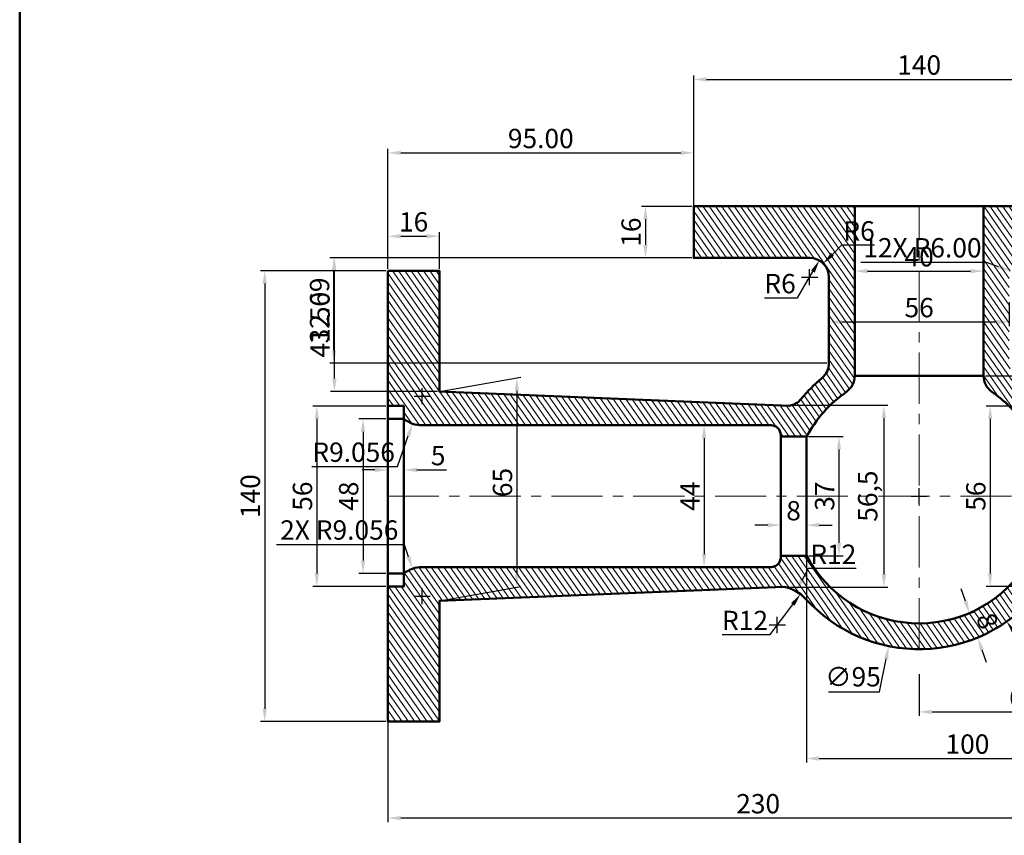
# Model space of a CAD drawing. Units: millimetres. Extents: x 39 to 520, y -165 to 464.
# Tile 2 of 4: x 39 to 345, y -9 to 244. Entities that reach past the tile are written whole.
import ezdxf

# ---------------------------------------------------------------- set-up
doc = ezdxf.new("R2010")
doc.units = ezdxf.units.MM
doc.header["$LTSCALE"] = 0.5
doc.linetypes.add('CENTER', pattern=[50.8, 31.75, -6.35, 6.35, -6.35])
for name, color, linetype, lineweight in [('M-CNTR', 1, 'CENTER', 18), ('M-DIMS', 2, 'Continuous', 25), ('M-HATC', 8, 'Continuous', 18), ('M-OUTL', 7, 'Continuous', 50), ('M-TTLB', 7, 'Continuous', 50)]:
    doc.layers.add(name, color=color, linetype=linetype, lineweight=lineweight)
doc.styles.get("Standard").update_dxf_attribs({"font": 'arial.ttf'})
doc.dimstyles.new('ISO-25', dxfattribs={"dimtxt": 6, "dimasz": 4, "dimexe": 1.25, "dimexo": 0.625, "dimtad": 1, "dimtoh": 1, "dimdec": 1, "dimtxsty": 'Standard', "dimcen": 2.5, "dimadec": 0, "dimazin": 0, "dimtfac": 1, "dimtdec": 1, "dimtofl": 0, "dimtmove": 0, "dimatfit": 3, "dimfxl": 1, "dimarcsym": 0})

# ---------------------------------------------------------------- blocks, each defined once
blk = doc.blocks.new('*D1')
at = {"layer": 'Defpoints', "color": 0, "ltscale": 0.5, "transparency": 16777216}
for p in [(388.62, 225.52), (248.62, 186.1), (388.62, 186.1)]:
    blk.add_point(p, dxfattribs=at)
at = {"layer": 'M-DIMS', "color": 0, "lineweight": -2, "ltscale": 0.5, "transparency": 16777216}
for p, q in [((248.62, 186.73), (248.62, 226.77)), ((388.62, 186.73), (388.62, 226.77)), ((252.62, 225.52), (384.62, 225.52))]:
    blk.add_line(p, q, dxfattribs=at)
at = {"layer": 'M-DIMS', "color": 0, "ltscale": 0.5, "transparency": 16777216}
for points in [[(252.62, 226.18), (252.62, 224.85), (248.62, 225.52)], [(384.62, 226.18), (384.62, 224.85), (388.62, 225.52)]]:
    blk.add_solid(points, dxfattribs=at)
at = {"layer": 'M-DIMS', "color": 0, "ltscale": 0.5, "transparency": 16777216, "insert": (318.62, 229.21), "char_height": 6, "attachment_point": 5}
blk.add_mtext('140', dxfattribs=at)
blk = doc.blocks.new('*D2')
at = {"layer": 'Defpoints', "color": 0, "ltscale": 0.5, "transparency": 16777216}
for p in [(290.62, 156.95), (346.62, 156.95), (346.62, 150.19)]:
    blk.add_point(p, dxfattribs=at)
at = {"layer": 'M-DIMS', "color": 0, "lineweight": -2, "ltscale": 0.5, "transparency": 16777216}
for p, q in [((290.62, 156.32), (290.62, 148.94)), ((346.62, 156.32), (346.62, 148.94)), ((294.62, 150.19), (342.62, 150.19))]:
    blk.add_line(p, q, dxfattribs=at)
at = {"layer": 'M-DIMS', "color": 0, "ltscale": 0.5, "transparency": 16777216}
for points in [[(294.62, 150.85), (294.62, 149.52), (290.62, 150.19)], [(342.62, 150.85), (342.62, 149.52), (346.62, 150.19)]]:
    blk.add_solid(points, dxfattribs=at)
at = {"layer": 'M-DIMS', "color": 0, "ltscale": 0.5, "transparency": 16777216, "insert": (318.62, 153.88), "char_height": 6, "attachment_point": 5}
blk.add_mtext('56', dxfattribs=at)
blk = doc.blocks.new('*D3')
at = {"layer": 'Defpoints', "color": 0, "ltscale": 0.5, "transparency": 16777216}
for p in [(298.62, 172.66), (338.62, 172.66), (338.62, 165.99)]:
    blk.add_point(p, dxfattribs=at)
at = {"layer": 'M-DIMS', "color": 0, "lineweight": -2, "ltscale": 0.5, "transparency": 16777216}
for p, q in [((298.62, 172.04), (298.62, 164.74)), ((338.62, 172.04), (338.62, 164.74)), ((302.62, 165.99), (334.62, 165.99))]:
    blk.add_line(p, q, dxfattribs=at)
at = {"layer": 'M-DIMS', "color": 0, "ltscale": 0.5, "transparency": 16777216}
for points in [[(302.62, 166.65), (302.62, 165.32), (298.62, 165.99)], [(334.62, 166.65), (334.62, 165.32), (338.62, 165.99)]]:
    blk.add_solid(points, dxfattribs=at)
at = {"layer": 'M-DIMS', "color": 0, "ltscale": 0.5, "transparency": 16777216, "insert": (318.62, 169.67), "char_height": 6, "attachment_point": 5}
blk.add_mtext('40', dxfattribs=at)
blk = doc.blocks.new('*D5')
at = {"layer": 'Defpoints', "color": 0, "ltscale": 0.5, "transparency": 16777216}
for p in [(248.62, 186.1), (233.62, 170.1), (248.62, 170.1)]:
    blk.add_point(p, dxfattribs=at)
at = {"layer": 'M-DIMS', "color": 0, "lineweight": -2, "ltscale": 0.5, "transparency": 16777216}
for p, q in [((248, 186.1), (232.37, 186.1)), ((233.62, 182.1), (233.62, 174.1)), ((248, 170.1), (232.37, 170.1))]:
    blk.add_line(p, q, dxfattribs=at)
at = {"layer": 'M-DIMS', "color": 0, "ltscale": 0.5, "transparency": 16777216}
for points in [[(232.96, 182.1), (234.29, 182.1), (233.62, 186.1)], [(232.96, 174.1), (234.29, 174.1), (233.62, 170.1)]]:
    blk.add_solid(points, dxfattribs=at)
at = {"layer": 'M-DIMS', "color": 0, "ltscale": 0.5, "transparency": 16777216, "insert": (229.94, 178.1), "char_height": 6, "attachment_point": 5, "rotation": 90}
blk.add_mtext('16', dxfattribs=at)
blk = doc.blocks.new('*D11')
at = {"layer": 'Defpoints', "color": 0, "ltscale": 0.5, "transparency": 16777216}
for p in [(318.62, 41.45), (383.62, 36.1), (383.62, 29.1)]:
    blk.add_point(p, dxfattribs=at)
at = {"layer": 'M-DIMS', "color": 0, "lineweight": -2, "ltscale": 0.5, "transparency": 16777216}
for p, q in [((318.62, 40.83), (318.62, 27.85)), ((383.62, 35.48), (383.62, 27.85)), ((322.62, 29.1), (379.62, 29.1))]:
    blk.add_line(p, q, dxfattribs=at)
at = {"layer": 'M-DIMS', "color": 0, "ltscale": 0.5, "transparency": 16777216}
for points in [[(322.62, 29.77), (322.62, 28.44), (318.62, 29.1)], [(379.62, 29.77), (379.62, 28.44), (383.62, 29.1)]]:
    blk.add_solid(points, dxfattribs=at)
at = {"layer": 'M-DIMS', "color": 0, "ltscale": 0.5, "transparency": 16777216, "insert": (351.12, 32.79), "char_height": 6, "attachment_point": 5}
blk.add_mtext('65', dxfattribs=at)
blk = doc.blocks.new('*D12')
at = {"layer": 'Defpoints', "color": 0, "ltscale": 0.5, "transparency": 16777216}
for p in [(283.62, 96.1), (383.62, 48.96), (383.62, 14.65)]:
    blk.add_point(p, dxfattribs=at)
at = {"layer": 'M-DIMS', "color": 0, "lineweight": -2, "ltscale": 0.5, "transparency": 16777216}
for p, q in [((283.62, 95.48), (283.62, 13.4)), ((383.62, 48.34), (383.62, 13.4)), ((287.62, 14.65), (379.62, 14.65))]:
    blk.add_line(p, q, dxfattribs=at)
at = {"layer": 'M-DIMS', "color": 0, "ltscale": 0.5, "transparency": 16777216}
for points in [[(287.62, 15.32), (287.62, 13.98), (283.62, 14.65)], [(379.62, 15.32), (379.62, 13.98), (383.62, 14.65)]]:
    blk.add_solid(points, dxfattribs=at)
at = {"layer": 'M-DIMS', "color": 0, "ltscale": 0.5, "transparency": 16777216, "insert": (333.62, 18.34), "char_height": 6, "attachment_point": 5}
blk.add_mtext('100', dxfattribs=at)
blk = doc.blocks.new('*D13')
at = {"layer": 'Defpoints', "color": 0, "ltscale": 0.5, "transparency": 16777216}
for p in [(153.62, 36.1), (383.62, 36.1), (153.62, -3.86)]:
    blk.add_point(p, dxfattribs=at)
at = {"layer": 'M-DIMS', "color": 0, "lineweight": -2, "ltscale": 0.5, "transparency": 16777216}
for p, q in [((153.62, 35.48), (153.62, -5.11)), ((383.62, 35.48), (383.62, -5.11)), ((379.62, -3.86), (157.62, -3.86))]:
    blk.add_line(p, q, dxfattribs=at)
at = {"layer": 'M-DIMS', "color": 0, "ltscale": 0.5, "transparency": 16777216}
for points in [[(157.62, -3.19), (157.62, -4.53), (153.62, -3.86)], [(379.62, -3.19), (379.62, -4.53), (383.62, -3.86)]]:
    blk.add_solid(points, dxfattribs=at)
at = {"layer": 'M-DIMS', "color": 0, "ltscale": 0.5, "transparency": 16777216, "insert": (268.62, -0.17), "char_height": 6, "attachment_point": 5}
blk.add_mtext('230', dxfattribs=at)
blk = doc.blocks.new('*D14')
at = {"layer": 'Defpoints', "color": 0, "ltscale": 0.5, "transparency": 16777216}
for p in [(359.93, 124.1), (340.68, 68.1), (362.28, 68.1)]:
    blk.add_point(p, dxfattribs=at)
at = {"layer": 'M-DIMS', "color": 0, "lineweight": -2, "ltscale": 0.5, "transparency": 16777216}
for p, q in [((359.3, 124.1), (339.43, 124.1)), ((340.68, 120.1), (340.68, 72.1)), ((361.65, 68.1), (339.43, 68.1))]:
    blk.add_line(p, q, dxfattribs=at)
at = {"layer": 'M-DIMS', "color": 0, "ltscale": 0.5, "transparency": 16777216}
for points in [[(340.02, 120.1), (341.35, 120.1), (340.68, 124.1)], [(340.02, 72.1), (341.35, 72.1), (340.68, 68.1)]]:
    blk.add_solid(points, dxfattribs=at)
at = {"layer": 'M-DIMS', "color": 0, "ltscale": 0.5, "transparency": 16777216, "insert": (337, 96.1), "char_height": 6, "attachment_point": 5, "rotation": 90}
blk.add_mtext('56', dxfattribs=at)
blk = doc.blocks.new('*D16')
at = {"layer": 'Defpoints', "color": 0, "ltscale": 0.5, "transparency": 16777216}
for p in [(283.62, 114.6), (283.72, 77.6), (293.73, 77.6)]:
    blk.add_point(p, dxfattribs=at)
at = {"layer": 'M-DIMS', "color": 0, "lineweight": -2, "ltscale": 0.5, "transparency": 16777216}
for p, q in [((284.25, 114.6), (294.98, 114.6)), ((293.73, 110.6), (293.73, 81.6)), ((284.35, 77.6), (294.98, 77.6))]:
    blk.add_line(p, q, dxfattribs=at)
at = {"layer": 'M-DIMS', "color": 0, "ltscale": 0.5, "transparency": 16777216}
for points in [[(293.07, 110.6), (294.4, 110.6), (293.73, 114.6)], [(293.07, 81.6), (294.4, 81.6), (293.73, 77.6)]]:
    blk.add_solid(points, dxfattribs=at)
at = {"layer": 'M-DIMS', "color": 0, "ltscale": 0.5, "transparency": 16777216, "insert": (290.04, 96.1), "char_height": 6, "attachment_point": 5, "rotation": 90}
blk.add_mtext('37', dxfattribs=at)
blk = doc.blocks.new('*D17')
at = {"layer": 'Defpoints', "color": 0, "ltscale": 0.5, "transparency": 16777216}
for p in [(275.62, 88.27), (275.62, 87.12), (283.62, 88.27)]:
    blk.add_point(p, dxfattribs=at)
at = {"layer": 'M-DIMS', "color": 0, "lineweight": -2, "ltscale": 0.5, "transparency": 16777216}
for p, q in [((271.62, 87.12), (267.62, 87.12)), ((275.62, 87.64), (275.62, 85.87)), ((283.62, 87.64), (283.62, 85.87)), ((287.62, 87.12), (291.62, 87.12))]:
    blk.add_line(p, q, dxfattribs=at)
at = {"layer": 'M-DIMS', "color": 0, "ltscale": 0.5, "transparency": 16777216}
for points in [[(271.62, 87.78), (271.62, 86.45), (275.62, 87.12)], [(287.62, 87.78), (287.62, 86.45), (283.62, 87.12)]]:
    blk.add_solid(points, dxfattribs=at)
at = {"layer": 'M-DIMS', "color": 0, "ltscale": 0.5, "transparency": 16777216, "insert": (279.62, 90.81), "char_height": 6, "attachment_point": 5}
blk.add_mtext('8', dxfattribs=at)
blk = doc.blocks.new('*D18')
at = {"layer": 'Defpoints', "color": 0, "ltscale": 0.5, "transparency": 16777216}
for p in [(274.95, 124.34), (275.62, 67.89), (307.66, 67.89)]:
    blk.add_point(p, dxfattribs=at)
at = {"layer": 'M-DIMS', "color": 0, "lineweight": -2, "ltscale": 0.5, "transparency": 16777216}
for p, q in [((275.57, 124.34), (308.91, 124.34)), ((307.66, 120.34), (307.66, 71.89)), ((276.25, 67.89), (308.91, 67.89))]:
    blk.add_line(p, q, dxfattribs=at)
at = {"layer": 'M-DIMS', "color": 0, "ltscale": 0.5, "transparency": 16777216}
for points in [[(306.99, 120.34), (308.32, 120.34), (307.66, 124.34)], [(306.99, 71.89), (308.32, 71.89), (307.66, 67.89)]]:
    blk.add_solid(points, dxfattribs=at)
at = {"layer": 'M-DIMS', "color": 0, "ltscale": 0.5, "transparency": 16777216, "insert": (303.43, 96.12), "char_height": 6, "attachment_point": 5, "rotation": 90}
blk.add_mtext('56,5', dxfattribs=at)
blk = doc.blocks.new('*D19')
at = {"layer": 'Defpoints', "color": 0, "ltscale": 0.5, "transparency": 16777216}
for p in [(169.62, 128.6), (193.67, 67.84), (169.62, 63.6)]:
    blk.add_point(p, dxfattribs=at)
at = {"layer": 'M-DIMS', "color": 0, "lineweight": -2, "ltscale": 0.5, "transparency": 16777216}
for p, q in [((170.25, 128.71), (194.92, 133.06)), ((193.67, 128.84), (193.67, 71.84)), ((170.25, 63.71), (194.92, 68.06))]:
    blk.add_line(p, q, dxfattribs=at)
at = {"layer": 'M-DIMS', "color": 0, "ltscale": 0.5, "transparency": 16777216}
for points in [[(193.01, 128.84), (194.34, 128.84), (193.67, 132.84)], [(193.01, 71.84), (194.34, 71.84), (193.67, 67.84)]]:
    blk.add_solid(points, dxfattribs=at)
at = {"layer": 'M-DIMS', "color": 0, "ltscale": 0.5, "transparency": 16777216, "insert": (189.99, 100.34), "char_height": 6, "attachment_point": 5, "rotation": 90}
blk.add_mtext('65', dxfattribs=at)
blk = doc.blocks.new('*D20')
at = {"layer": 'Defpoints', "color": 0, "ltscale": 0.5, "transparency": 16777216}
for p in [(250.84, 118.1), (250.84, 74.1), (251.84, 74.1)]:
    blk.add_point(p, dxfattribs=at)
at = {"layer": 'M-DIMS', "color": 0, "lineweight": -2, "ltscale": 0.5, "transparency": 16777216}
for p, q in [((251.47, 118.1), (253.09, 118.1)), ((251.84, 114.1), (251.84, 78.1)), ((251.47, 74.1), (253.09, 74.1))]:
    blk.add_line(p, q, dxfattribs=at)
at = {"layer": 'M-DIMS', "color": 0, "ltscale": 0.5, "transparency": 16777216}
for points in [[(251.17, 114.1), (252.5, 114.1), (251.84, 118.1)], [(251.17, 78.1), (252.5, 78.1), (251.84, 74.1)]]:
    blk.add_solid(points, dxfattribs=at)
at = {"layer": 'M-DIMS', "color": 0, "ltscale": 0.5, "transparency": 16777216, "insert": (248.21, 96.1), "char_height": 6, "attachment_point": 5, "rotation": 90}
blk.add_mtext('44', dxfattribs=at)
blk = doc.blocks.new('*D21')
at = {"layer": 'Defpoints', "color": 0, "ltscale": 0.5, "transparency": 16777216}
for p in [(153.62, 166.1), (115.36, 26.1), (153.62, 26.1)]:
    blk.add_point(p, dxfattribs=at)
at = {"layer": 'M-DIMS', "color": 0, "lineweight": -2, "ltscale": 0.5, "transparency": 16777216}
for p, q in [((153, 166.1), (114.11, 166.1)), ((115.36, 162.1), (115.36, 30.1)), ((153, 26.1), (114.11, 26.1))]:
    blk.add_line(p, q, dxfattribs=at)
at = {"layer": 'M-DIMS', "color": 0, "ltscale": 0.5, "transparency": 16777216}
for points in [[(114.7, 162.1), (116.03, 162.1), (115.36, 166.1)], [(114.7, 30.1), (116.03, 30.1), (115.36, 26.1)]]:
    blk.add_solid(points, dxfattribs=at)
at = {"layer": 'M-DIMS', "color": 0, "ltscale": 0.5, "transparency": 16777216, "insert": (111.67, 96.1), "char_height": 6, "attachment_point": 5, "rotation": 90}
blk.add_mtext('140', dxfattribs=at)
blk = doc.blocks.new('*D22')
at = {"layer": 'Defpoints', "color": 0, "ltscale": 0.5, "transparency": 16777216}
for p in [(153.62, 120.1), (145.9, 72.1), (153.62, 72.1)]:
    blk.add_point(p, dxfattribs=at)
at = {"layer": 'M-DIMS', "color": 0, "lineweight": -2, "ltscale": 0.5, "transparency": 16777216}
for p, q in [((153, 120.1), (144.65, 120.1)), ((145.9, 116.1), (145.9, 76.1)), ((153, 72.1), (144.65, 72.1))]:
    blk.add_line(p, q, dxfattribs=at)
at = {"layer": 'M-DIMS', "color": 0, "ltscale": 0.5, "transparency": 16777216}
for points in [[(145.23, 116.1), (146.57, 116.1), (145.9, 120.1)], [(145.23, 76.1), (146.57, 76.1), (145.9, 72.1)]]:
    blk.add_solid(points, dxfattribs=at)
at = {"layer": 'M-DIMS', "color": 0, "ltscale": 0.5, "transparency": 16777216, "insert": (142.21, 96.1), "char_height": 6, "attachment_point": 5, "rotation": 90}
blk.add_mtext('48', dxfattribs=at)
blk = doc.blocks.new('*D23')
at = {"layer": 'Defpoints', "color": 0, "ltscale": 0.5, "transparency": 16777216}
for p in [(153.62, 124.1), (131.56, 68.1), (153.62, 68.1)]:
    blk.add_point(p, dxfattribs=at)
at = {"layer": 'M-DIMS', "color": 0, "lineweight": -2, "ltscale": 0.5, "transparency": 16777216}
for p, q in [((153, 124.1), (130.31, 124.1)), ((131.56, 120.1), (131.56, 72.1)), ((153, 68.1), (130.31, 68.1))]:
    blk.add_line(p, q, dxfattribs=at)
at = {"layer": 'M-DIMS', "color": 0, "ltscale": 0.5, "transparency": 16777216}
for points in [[(130.9, 120.1), (132.23, 120.1), (131.56, 124.1)], [(130.9, 72.1), (132.23, 72.1), (131.56, 68.1)]]:
    blk.add_solid(points, dxfattribs=at)
at = {"layer": 'M-DIMS', "color": 0, "ltscale": 0.5, "transparency": 16777216, "insert": (127.87, 96.1), "char_height": 6, "attachment_point": 5, "rotation": 90}
blk.add_mtext('56', dxfattribs=at)
blk = doc.blocks.new('*D24')
at = {"layer": 'Defpoints', "color": 0, "ltscale": 0.5, "transparency": 16777216}
for p in [(153.62, 104.33), (158.62, 104.33), (158.62, 104.25)]:
    blk.add_point(p, dxfattribs=at)
at = {"layer": 'M-DIMS', "color": 0, "lineweight": -2, "ltscale": 0.5, "transparency": 16777216}
for p, q in [((149.62, 104.25), (145.62, 104.25)), ((162.62, 104.25), (171.85, 104.25)), ((153.62, 103.71), (153.62, 103)), ((158.62, 103.71), (158.62, 103))]:
    blk.add_line(p, q, dxfattribs=at)
at = {"layer": 'M-DIMS', "color": 0, "ltscale": 0.5, "transparency": 16777216}
for points in [[(149.62, 104.92), (149.62, 103.59), (153.62, 104.25)], [(162.62, 104.92), (162.62, 103.59), (158.62, 104.25)]]:
    blk.add_solid(points, dxfattribs=at)
at = {"layer": 'M-DIMS', "color": 0, "ltscale": 0.5, "transparency": 16777216, "insert": (169.24, 107.93), "char_height": 6, "attachment_point": 5}
blk.add_mtext('5', dxfattribs=at)
blk = doc.blocks.new('*D25')
at = {"layer": 'Defpoints', "color": 0, "ltscale": 0.5, "transparency": 16777216}
for p in [(169.62, 176.82), (153.62, 166.1), (169.62, 166.1)]:
    blk.add_point(p, dxfattribs=at)
at = {"layer": 'M-DIMS', "color": 0, "lineweight": -2, "ltscale": 0.5, "transparency": 16777216}
for p, q in [((153.62, 166.73), (153.62, 178.07)), ((169.62, 166.73), (169.62, 178.07)), ((157.62, 176.82), (165.62, 176.82))]:
    blk.add_line(p, q, dxfattribs=at)
at = {"layer": 'M-DIMS', "color": 0, "ltscale": 0.5, "transparency": 16777216}
for points in [[(157.62, 177.48), (157.62, 176.15), (153.62, 176.82)], [(165.62, 177.48), (165.62, 176.15), (169.62, 176.82)]]:
    blk.add_solid(points, dxfattribs=at)
at = {"layer": 'M-DIMS', "color": 0, "ltscale": 0.5, "transparency": 16777216, "insert": (161.62, 180.51), "char_height": 6, "attachment_point": 5}
blk.add_mtext('16', dxfattribs=at)
blk = doc.blocks.new('*D26')
at = {"layer": 'Defpoints', "color": 0, "ltscale": 0.5, "transparency": 16777216}
for p in [(328.07, 142.65), (309.17, 49.55)]:
    blk.add_point(p, dxfattribs=at)
at = {"layer": 'M-DIMS', "color": 0, "lineweight": -2, "ltscale": 0.5, "transparency": 16777216}
for p, q in [((318.62, 93.6), (318.62, 98.6)), ((316.12, 96.1), (321.12, 96.1)), ((306.3, 35.38), (308.38, 45.63)), ((290.5, 35.38), (306.3, 35.38))]:
    blk.add_line(p, q, dxfattribs=at)
at = {"layer": 'M-DIMS', "color": 0, "ltscale": 0.5, "transparency": 16777216}
blk.add_solid([(307.73, 45.76), (309.03, 45.5), (309.17, 49.55)], dxfattribs=at)
at = {"layer": 'M-DIMS', "color": 0, "ltscale": 0.5, "transparency": 16777216, "insert": (298.09, 39.24), "char_height": 6, "attachment_point": 5}
blk.add_mtext('∅95', dxfattribs=at)
blk = doc.blocks.new('*D27')
at = {"layer": 'Defpoints', "color": 0, "ltscale": 0.5, "transparency": 16777216}
for p in [(331.31, 58.7), (336.86, 52.13), (333.88, 51.12)]:
    blk.add_point(p, dxfattribs=at)
at = {"layer": 'M-DIMS', "color": 0, "lineweight": -2, "ltscale": 0.5, "transparency": 16777216}
for p, q in [((333, 63.49), (331.72, 67.28)), ((331.9, 58.9), (335.47, 60.11)), ((334.47, 51.32), (338.04, 52.53)), ((338.14, 48.34), (339.42, 44.55))]:
    blk.add_line(p, q, dxfattribs=at)
at = {"layer": 'M-DIMS', "color": 0, "ltscale": 0.5, "transparency": 16777216}
for points in [[(333.63, 63.71), (332.37, 63.28), (334.29, 59.71)], [(338.77, 48.56), (337.51, 48.13), (336.86, 52.13)]]:
    blk.add_solid(points, dxfattribs=at)
at = {"layer": 'M-DIMS', "color": 0, "ltscale": 0.5, "transparency": 16777216, "insert": (339.06, 57.1), "char_height": 6, "attachment_point": 5, "rotation": 288.7308}
blk.add_mtext('8', dxfattribs=at)
blk = doc.blocks.new('*D28')
at = {"layer": 'Defpoints', "color": 0, "ltscale": 0.5, "transparency": 16777216}
for p in [(287.62, 169.3), (284.62, 164.1)]:
    blk.add_point(p, dxfattribs=at)
at = {"layer": 'M-DIMS', "color": 0, "lineweight": -2, "ltscale": 0.5, "transparency": 16777216}
for p, q in [((280.89, 157.64), (285.62, 165.84)), ((270.6, 157.64), (280.89, 157.64))]:
    blk.add_line(p, q, dxfattribs=at)
at = {"layer": 'M-DIMS', "color": 0, "ltscale": 0.5, "transparency": 16777216}
blk.add_solid([(285.05, 166.17), (286.2, 165.5), (287.62, 169.3)], dxfattribs=at)
at = {"layer": 'M-DIMS', "color": 0, "ltscale": 0.5, "transparency": 16777216, "insert": (275.43, 161.33), "char_height": 6, "attachment_point": 5}
blk.add_mtext('R6', dxfattribs=at)
blk = doc.blocks.new('*D29')
at = {"layer": 'Defpoints', "color": 0, "ltscale": 0.5, "transparency": 16777216}
for p in [(281.79, 65.69), (274.57, 56.1)]:
    blk.add_point(p, dxfattribs=at)
at = {"layer": 'M-DIMS', "color": 0, "lineweight": -2, "ltscale": 0.5, "transparency": 16777216}
for p, q in [((272.31, 53.1), (279.39, 62.49)), ((257.41, 53.1), (272.31, 53.1))]:
    blk.add_line(p, q, dxfattribs=at)
at = {"layer": 'M-DIMS', "color": 0, "ltscale": 0.5, "transparency": 16777216}
blk.add_solid([(278.85, 62.9), (279.92, 62.09), (281.79, 65.69)], dxfattribs=at)
at = {"layer": 'M-DIMS', "color": 0, "ltscale": 0.5, "transparency": 16777216, "insert": (264.55, 56.73), "char_height": 6, "attachment_point": 5}
blk.add_mtext('R12', dxfattribs=at)
blk = doc.blocks.new('*D58')
at = {"layer": 'Defpoints', "color": 0, "ltscale": 0.5, "transparency": 16777216}
for p in [(338.62, 186.1), (405.37, 186.1), (338.62, 133.44)]:
    blk.add_point(p, dxfattribs=at)
at = {"layer": 'M-DIMS', "color": 0, "lineweight": -2, "ltscale": 0.5, "transparency": 16777216}
for p, q in [((339.25, 186.1), (406.62, 186.1)), ((405.37, 137.44), (405.37, 182.1)), ((339.25, 133.44), (406.62, 133.44))]:
    blk.add_line(p, q, dxfattribs=at)
at = {"layer": 'M-DIMS', "color": 0, "ltscale": 0.5, "transparency": 16777216}
for points in [[(404.71, 182.1), (406.04, 182.1), (405.37, 186.1)], [(404.71, 137.44), (406.04, 137.44), (405.37, 133.44)]]:
    blk.add_solid(points, dxfattribs=at)
at = {"layer": 'M-DIMS', "color": 0, "ltscale": 0.5, "transparency": 16777216, "insert": (401.68, 159.77), "char_height": 6, "attachment_point": 5, "rotation": 90}
blk.add_mtext('52.66', dxfattribs=at)
blk = doc.blocks.new('*D59')
at = {"layer": 'Defpoints', "color": 0, "ltscale": 0.5, "transparency": 16777216}
for p in [(136.87, 170.1), (248.62, 170.1), (290.62, 137.41)]:
    blk.add_point(p, dxfattribs=at)
at = {"layer": 'M-DIMS', "color": 0, "lineweight": -2, "ltscale": 0.5, "transparency": 16777216}
for p, q in [((248, 170.1), (135.62, 170.1)), ((136.87, 141.41), (136.87, 166.1)), ((290, 137.41), (135.62, 137.41))]:
    blk.add_line(p, q, dxfattribs=at)
at = {"layer": 'M-DIMS', "color": 0, "ltscale": 0.5, "transparency": 16777216}
for points in [[(136.21, 166.1), (137.54, 166.1), (136.87, 170.1)], [(136.21, 141.41), (137.54, 141.41), (136.87, 137.41)]]:
    blk.add_solid(points, dxfattribs=at)
at = {"layer": 'M-DIMS', "color": 0, "ltscale": 0.5, "transparency": 16777216, "insert": (133.18, 153.76), "char_height": 6, "attachment_point": 5, "rotation": 90}
blk.add_mtext('32.69', dxfattribs=at)
blk = doc.blocks.new('*D60')
at = {"layer": 'Defpoints', "color": 0, "ltscale": 0.5, "transparency": 16777216}
for p in [(288.86, 168.36), (284.62, 164.1)]:
    blk.add_point(p, dxfattribs=at)
at = {"layer": 'M-DIMS', "color": 0, "lineweight": -2, "ltscale": 0.5, "transparency": 16777216}
for p, q in [((294.5, 174.03), (291.68, 171.19)), ((304.8, 174.03), (294.5, 174.03)), ((284.62, 161.6), (284.62, 166.6)), ((282.12, 164.1), (287.12, 164.1))]:
    blk.add_line(p, q, dxfattribs=at)
at = {"layer": 'M-DIMS', "color": 0, "ltscale": 0.5, "transparency": 16777216}
blk.add_solid([(291.21, 171.66), (292.15, 170.72), (288.86, 168.36)], dxfattribs=at)
at = {"layer": 'M-DIMS', "color": 0, "ltscale": 0.5, "transparency": 16777216, "insert": (299.96, 177.71), "char_height": 6, "attachment_point": 5}
blk.add_mtext('R6', dxfattribs=at)
blk = doc.blocks.new('*D61')
at = {"layer": 'Defpoints', "color": 0, "ltscale": 0.5, "transparency": 16777216}
for p in [(280.35, 66.62), (274.57, 56.1)]:
    blk.add_point(p, dxfattribs=at)
at = {"layer": 'M-DIMS', "color": 0, "lineweight": -2, "ltscale": 0.5, "transparency": 16777216}
for p, q in [((284.19, 73.64), (282.27, 70.13)), ((299.09, 73.64), (284.19, 73.64)), ((274.57, 53.6), (274.57, 58.6)), ((272.07, 56.1), (277.07, 56.1))]:
    blk.add_line(p, q, dxfattribs=at)
at = {"layer": 'M-DIMS', "color": 0, "ltscale": 0.5, "transparency": 16777216}
blk.add_solid([(281.68, 70.45), (282.85, 69.81), (280.35, 66.62)], dxfattribs=at)
at = {"layer": 'M-DIMS', "color": 0, "ltscale": 0.5, "transparency": 16777216, "insert": (291.96, 77.28), "char_height": 6, "attachment_point": 5}
blk.add_mtext('R12', dxfattribs=at)
blk = doc.blocks.new('*D63')
at = {"layer": 'Defpoints', "color": 0, "ltscale": 0.5, "transparency": 16777216}
for p in [(164.3, 127.16), (161.29, 118.62)]:
    blk.add_point(p, dxfattribs=at)
at = {"layer": 'M-DIMS', "color": 0, "lineweight": -2, "ltscale": 0.5, "transparency": 16777216}
for p, q in [((164.3, 124.66), (164.3, 129.66)), ((161.8, 127.16), (166.8, 127.16)), ((156.61, 105.29), (159.97, 114.84)), ((130, 105.29), (156.61, 105.29))]:
    blk.add_line(p, q, dxfattribs=at)
at = {"layer": 'M-DIMS', "color": 0, "ltscale": 0.5, "transparency": 16777216}
blk.add_solid([(159.34, 115.06), (160.6, 114.62), (161.29, 118.62)], dxfattribs=at)
at = {"layer": 'M-DIMS', "color": 0, "ltscale": 0.5, "transparency": 16777216, "insert": (142.99, 108.98), "char_height": 6, "attachment_point": 5}
blk.add_mtext('R9.056', dxfattribs=at)
blk = doc.blocks.new('*D64')
at = {"layer": 'Defpoints', "color": 0, "ltscale": 0.5, "transparency": 16777216}
for p in [(291.42, 135.04), (345.83, 57.16)]:
    blk.add_point(p, dxfattribs=at)
at = {"layer": 'M-DIMS', "color": 0, "lineweight": -2, "ltscale": 0.5, "transparency": 16777216}
for p, q in [((318.62, 93.6), (318.62, 98.6)), ((316.12, 96.1), (321.12, 96.1)), ((362.15, 33.8), (348.12, 53.88)), ((377.94, 33.8), (362.15, 33.8))]:
    blk.add_line(p, q, dxfattribs=at)
at = {"layer": 'M-DIMS', "color": 0, "ltscale": 0.5, "transparency": 16777216}
blk.add_solid([(348.66, 54.27), (347.57, 53.5), (345.83, 57.16)], dxfattribs=at)
at = {"layer": 'M-DIMS', "color": 0, "ltscale": 0.5, "transparency": 16777216, "insert": (370.36, 37.66), "char_height": 6, "attachment_point": 5}
blk.add_mtext('∅95', dxfattribs=at)
blk = doc.blocks.new('*D67')
at = {"layer": 'Defpoints', "color": 0, "ltscale": 0.5, "transparency": 16777216}
for p in [(248.62, 202.7), (248.62, 170.1), (153.62, 166.1)]:
    blk.add_point(p, dxfattribs=at)
at = {"layer": 'M-DIMS', "color": 0, "lineweight": -2, "ltscale": 0.5, "transparency": 16777216}
for p, q in [((153.62, 166.73), (153.62, 203.95)), ((157.62, 202.7), (244.62, 202.7)), ((248.62, 170.73), (248.62, 203.95))]:
    blk.add_line(p, q, dxfattribs=at)
at = {"layer": 'M-DIMS', "color": 0, "ltscale": 0.5, "transparency": 16777216}
for points in [[(157.62, 203.37), (157.62, 202.04), (153.62, 202.7)], [(244.62, 203.37), (244.62, 202.04), (248.62, 202.7)]]:
    blk.add_solid(points, dxfattribs=at)
at = {"layer": 'M-DIMS', "color": 0, "ltscale": 0.5, "transparency": 16777216, "insert": (201.12, 206.39), "char_height": 6, "attachment_point": 5}
blk.add_mtext('95.00', dxfattribs=at)
blk = doc.blocks.new('*D68')
at = {"layer": 'Defpoints', "color": 0, "ltscale": 0.5, "transparency": 16777216}
for p in [(137.02, 170.1), (248.62, 170.1), (169.62, 128.6)]:
    blk.add_point(p, dxfattribs=at)
at = {"layer": 'M-DIMS', "color": 0, "lineweight": -2, "ltscale": 0.5, "transparency": 16777216}
for p, q in [((248, 170.1), (135.77, 170.1)), ((137.02, 132.6), (137.02, 166.1)), ((169, 128.6), (135.77, 128.6))]:
    blk.add_line(p, q, dxfattribs=at)
at = {"layer": 'M-DIMS', "color": 0, "ltscale": 0.5, "transparency": 16777216}
for points in [[(136.36, 166.1), (137.69, 166.1), (137.02, 170.1)], [(136.36, 132.6), (137.69, 132.6), (137.02, 128.6)]]:
    blk.add_solid(points, dxfattribs=at)
at = {"layer": 'M-DIMS', "color": 0, "ltscale": 0.5, "transparency": 16777216, "insert": (133.33, 149.35), "char_height": 6, "attachment_point": 5, "rotation": 90}
blk.add_mtext('41.50', dxfattribs=at)
blk = doc.blocks.new('*D69')
at = {"layer": 'Defpoints', "color": 0, "ltscale": 0.5, "transparency": 16777216}
for p in [(346.97, 166.1), (352.62, 164.1)]:
    blk.add_point(p, dxfattribs=at)
at = {"layer": 'M-DIMS', "color": 0, "lineweight": -2, "ltscale": 0.5, "transparency": 16777216}
for p, q in [((300.5, 168.77), (339.42, 168.77)), ((339.42, 168.77), (343.19, 167.44)), ((352.62, 161.6), (352.62, 166.6)), ((350.12, 164.1), (355.12, 164.1))]:
    blk.add_line(p, q, dxfattribs=at)
at = {"layer": 'M-DIMS', "color": 0, "ltscale": 0.5, "transparency": 16777216}
blk.add_solid([(343.42, 168.06), (342.97, 166.81), (346.97, 166.1)], dxfattribs=at)
at = {"layer": 'M-DIMS', "color": 0, "ltscale": 0.5, "transparency": 16777216, "insert": (319.65, 172.46), "char_height": 6, "attachment_point": 5}
blk.add_mtext('12X R6.00', dxfattribs=at)
blk = doc.blocks.new('*D70')
at = {"layer": 'Defpoints', "color": 0, "ltscale": 0.5, "transparency": 16777216}
for p in [(161.29, 73.59), (164.3, 65.05)]:
    blk.add_point(p, dxfattribs=at)
at = {"layer": 'M-DIMS', "color": 0, "lineweight": -2, "ltscale": 0.5, "transparency": 16777216}
for p, q in [((119.03, 81.14), (158.64, 81.14)), ((158.64, 81.14), (159.97, 77.36)), ((164.3, 62.55), (164.3, 67.55)), ((161.8, 65.05), (166.8, 65.05))]:
    blk.add_line(p, q, dxfattribs=at)
at = {"layer": 'M-DIMS', "color": 0, "ltscale": 0.5, "transparency": 16777216}
blk.add_solid([(160.59, 77.58), (159.34, 77.14), (161.29, 73.59)], dxfattribs=at)
at = {"layer": 'M-DIMS', "color": 0, "ltscale": 0.5, "transparency": 16777216, "insert": (138.52, 84.82), "char_height": 6, "attachment_point": 5}
blk.add_mtext('2X R9.056', dxfattribs=at)

msp = doc.modelspace()

# ---------------------------------------------------------------- hatches: boundary and pattern name
at = {"layer": 'M-HATC', "ltscale": 0.5}
h = msp.add_hatch(dxfattribs=at)
h.set_pattern_fill('ANSI31', color=256, scale=0.5, angle=80)
h.paths.add_polyline_path([(296.0512, 128.5189, 0.24539268), (298.6226, 133.4428), (298.6226, 186.1031), (248.6226, 186.1031), (248.6226, 170.1031), (284.6226, 170.1031, -0.41421356), (290.6226, 164.1031), (290.6226, 137.4099, -0.22417658), (288.4357, 132.7774, 0.04839978), (281.9483, 126.29, -0.17668241), (278.4054, 124.2029), (169.6226, 128.6031), (169.6226, 166.1031), (153.6226, 166.1031), (153.6226, 124.1031), (158.6226, 124.1031), (158.6226, 120.1031, 0.17132661), (164.3106, 118.1031), (272.6226, 118.1031, -0.41421356), (275.6226, 115.1031), (275.6226, 114.6031), (283.7227, 114.6031, -0.11934263)])
h.paths.add_polyline_path([(283.7227, 77.6031), (275.6226, 77.6031), (275.6226, 77.1031, -0.41421356), (272.6226, 74.1031), (164.2881, 74.1031, 0.17068716), (158.6226, 72.1031), (158.6226, 68.1031), (153.6226, 68.1031), (153.6226, 26.1031), (169.6226, 26.1031), (169.6226, 63.6031), (276.6027, 67.9304, -0.16745848), (283.458, 64.1703, 0.21145125), (318.6226, 48.6031), (318.6226, 56.6031, -0.27766509)])
h.paths.add_polyline_path([(355.2968, 65.9162, -0.22417658), (359.9294, 68.1031), (364.6226, 68.1031, -0.41421356), (367.6226, 65.1031), (367.6226, 36.1031), (383.6226, 36.1031), (383.6226, 71.1031), (378.6226, 71.1031), (378.6226, 74.1031), (376.6226, 76.1031), (355.9622, 76.1031, 0.24539268), (351.0383, 73.5317, -0.24539268), (318.6226, 56.6031), (318.6226, 48.6031, 0.22417658)])
h.paths.add_polyline_path([(383.6226, 156.1031), (367.6226, 156.1031), (367.6226, 127.1031, -0.41421356), (364.6226, 124.1031), (359.9294, 124.1031, -0.22417658), (355.2968, 126.29, 0.04839978), (348.8095, 132.7774, -0.22417658), (346.6226, 137.4099), (346.6226, 164.1031, -0.41421356), (352.6226, 170.1031), (388.6226, 170.1031), (388.6226, 186.1031), (338.6226, 186.1031), (338.6226, 133.4428, 0.24539268), (341.194, 128.5189, -0.08880867), (351.0383, 118.6745, 0.24539268), (355.9622, 116.1031), (376.6226, 116.1031), (378.6226, 118.1031), (378.6226, 121.1031), (383.6226, 121.1031)])

# ---------------------------------------------------------------- linework, layer by layer
at = {"layer": 'M-CNTR'}
for p, q in [((318.6226, 48.6031), (318.6226, 186.1031)), ((153.6226, 96.1031), (383.6226, 96.1031))]:
    msp.add_line(p, q, dxfattribs=at)
at = {"layer": 'M-OUTL'}
for p, q in [((388.6226, 186.1031), (248.6226, 186.1031)), ((153.6226, 124.1031), (158.6226, 124.1031)), ((158.6226, 124.1031), (158.6226, 120.1031)), ((158.6226, 120.1031), (153.6226, 120.1031)), ((153.6226, 120.1031), (153.6226, 96.1031)), ((283.6226, 77.6031), (283.6226, 114.6031)), ((275.6226, 77.6031), (283.7227, 77.6031))]:
    msp.add_line(p, q, dxfattribs=at)
at = {"layer": 'M-OUTL', "ltscale": 0.5}
msp.add_line((298.6226, 133.4428), (338.6226, 133.4428), dxfattribs=at)
at = {"layer": 'M-OUTL'}
for points in [[(248.6226, 186.1031), (248.6226, 170.1031), (284.6226, 170.1031, -0.41421356), (290.6226, 164.1031), (290.6226, 137.4099, -0.22417658), (288.4357, 132.7774, 0.04839978), (281.9483, 126.29, -0.17668241), (278.4054, 124.2029), (169.6226, 128.6031), (169.6226, 166.1031), (153.6226, 166.1031)], [(283.6226, 114.4129, -0.12072251), (296.0512, 128.5189, 0.24539268), (298.6226, 133.4428), (298.6226, 186.1031)], [(338.6226, 186.1031), (338.6226, 133.4428, 0.24539268), (341.194, 128.5189, -0.08880867), (351.0383, 118.6745, 0.24539268), (355.9622, 116.1031), (376.6226, 116.1031)], [(153.6226, 166.1031), (153.6226, 26.1031), (169.6226, 26.1031), (169.6226, 63.6031), (276.6027, 67.9304, -0.16745848), (283.458, 64.1703, 0.4573052), (355.2968, 65.9162, -0.22417658), (359.9294, 68.1031), (364.6226, 68.1031, -0.41421356), (367.6226, 65.1031), (367.6226, 36.1031), (383.6226, 36.1031), (383.6226, 96.1031)], [(164.2881, 74.1031), (272.6226, 74.1031, 0.41421356), (275.6226, 77.1031), (275.6226, 115.1031, 0.41421356), (272.6226, 118.1031), (164.2881, 118.1031)], [(283.6226, 77.7933, 0.5630935), (351.0383, 73.5317, -0.24539268), (355.9622, 76.1031), (376.6226, 76.1031)]]:
    msp.add_lwpolyline(points, format="xyb", dxfattribs=at)
at = {"layer": 'M-OUTL', "ltscale": 0.5}
for points in [[(153.6226, 68.1031), (158.6226, 68.1031), (158.6226, 120.1031, 0.17132661), (164.3106, 118.1031)], [(164.3106, 74.1031, 0.17132661), (158.6226, 72.1031), (153.6226, 72.1031)]]:
    msp.add_lwpolyline(points, format="xyb", dxfattribs=at)
at = {"layer": 'M-OUTL'}
msp.add_lwpolyline([(283.6226, 96.1031), (283.6226, 114.6031), (275.6226, 114.6031)], dxfattribs=at)
at = {"layer": 'M-TTLB', "ltscale": 0.5}
msp.add_lwpolyline([(39.27, 463.9335), (519.8288, 463.9335), (519.8288, -165.0878), (39.27, -165.0878)], close=True, dxfattribs=at)

# ---------------------------------------------------------------- dimensions: what is measured, and where the dimension line sits
at = {"layer": 'M-DIMS', "ltscale": 0.5}
for base, p1, p2, override, picture, middle in [((388.6226, 225.517), (248.6226, 186.1031), (388.6226, 186.1031), {"dimclrd": 0, "dimclre": 0, "dimclrt": 0}, '*D1', (318.6226, 229.2054)), ((248.6226, 202.7031), (153.6226, 166.1031), (248.6226, 170.1031), {"dimdec": 2, "dimlfac": 1, "dimrnd": 0, "dimzin": 0, "dimdsep": 46, "dimlunit": 2}, '*D67', (201.1226, 206.3916)), ((169.6226, 176.8174), (153.6226, 166.1031), (169.6226, 166.1031), {"dimclrd": 0, "dimclre": 0, "dimclrt": 0}, '*D25', (161.6226, 180.5058)), ((338.6226, 165.9859), (298.6226, 172.6626), (338.6226, 172.6626), {"dimclrd": 0, "dimclre": 0, "dimclrt": 0}, '*D3', (318.6226, 169.6743)), ((346.6226, 150.1873), (290.6226, 156.9452), (346.6226, 156.9452), {"dimclrd": 0, "dimclre": 0, "dimclrt": 0}, '*D2', (318.6226, 153.8757)), ((158.6226, 104.2536), (153.6226, 104.3334), (158.6226, 104.3334), {"dimclrd": 0, "dimclre": 0, "dimclrt": 0}, '*D24', (169.2367, 107.9298)), ((383.6226, 14.6514), (283.6226, 96.1031), (383.6226, 48.9607), {"dimclrd": 0, "dimclre": 0, "dimclrt": 0}, '*D12', (333.6226, 18.3398)), ((275.6226, 87.1167), (283.6226, 88.2653), (275.6226, 88.2653), {"dimclrd": 0, "dimclre": 0, "dimclrt": 0}, '*D17', (279.6226, 90.8051)), ((383.6226, 29.1036), (318.6226, 41.4507), (383.6226, 36.1031), {"dimclrd": 0, "dimclre": 0, "dimclrt": 0}, '*D11', (351.1226, 32.7921)), ((153.6226, -3.8615), (383.6226, 36.1031), (153.6226, 36.1031), {"dimclrd": 0, "dimclre": 0, "dimclrt": 0}, '*D13', (268.6226, -0.171))]:
    dim = msp.add_linear_dim(base=base, p1=p1, p2=p2, dimstyle='ISO-25', override=override, dxfattribs=at)
    dim.commit()
    dim.dimension.update_dxf_attribs({"geometry": picture, "text_midpoint": middle})
for base, p1, p2, override, picture, middle in [((233.6241, 170.1031), (248.6226, 186.1031), (248.6226, 170.1031), {"dimclrd": 0, "dimclre": 0, "dimclrt": 0}, '*D5', (229.9357, 178.1031)), ((405.3726, 186.1031), (338.6226, 133.4428), (338.6226, 186.1031), {"dimdec": 2, "dimlfac": 1, "dimrnd": 0, "dimzin": 0, "dimdsep": 46, "dimlunit": 2}, '*D58', (401.6842, 159.7729)), ((136.8726, 170.1031), (290.6226, 137.4099), (248.6226, 170.1031), {"dimdec": 2, "dimlfac": 1, "dimrnd": 0, "dimzin": 0, "dimdsep": 46, "dimlunit": 2}, '*D59', (133.1821, 153.7565)), ((137.0226, 170.1031), (169.6226, 128.6031), (248.6226, 170.1031), {"dimdec": 2, "dimlfac": 1, "dimrnd": 0, "dimzin": 0, "dimdsep": 46, "dimlunit": 2}, '*D68', (133.3342, 149.3531)), ((115.3625, 26.1031), (153.6226, 166.1031), (153.6226, 26.1031), {"dimclrd": 0, "dimclre": 0, "dimclrt": 0}, '*D21', (111.674, 96.1031)), ((193.6748, 67.8442), (169.6226, 128.6031), (169.6226, 63.6031), {"dimclrd": 0, "dimclre": 0, "dimclrt": 0}, '*D19', (189.9864, 100.3442)), ((131.5624, 68.1031), (153.6226, 124.1031), (153.6226, 68.1031), {"dimclrd": 0, "dimclre": 0, "dimclrt": 0}, '*D23', (127.8739, 96.1031)), ((307.656, 67.8908), (274.9474, 124.3428), (275.6226, 67.8908), {"dimclrd": 0, "dimclre": 0, "dimclrt": 0}, '*D18', (303.4253, 96.1168)), ((340.6837, 68.1031), (359.9294, 124.1031), (362.276, 68.1031), {"dimclrd": 0, "dimclre": 0, "dimclrt": 0}, '*D14', (336.9953, 96.1031)), ((145.8994, 72.1031), (153.6226, 120.1031), (153.6226, 72.1031), {"dimclrd": 0, "dimclre": 0, "dimclrt": 0}, '*D22', (142.211, 96.1031)), ((251.8355, 74.1031), (250.842, 118.1031), (250.842, 74.1031), {"dimclrd": 0, "dimclre": 0, "dimclrt": 0}, '*D20', (248.2105, 96.1031)), ((293.7319, 77.6031), (283.6226, 114.6031), (283.7227, 77.6031), {"dimclrd": 0, "dimclre": 0, "dimclrt": 0}, '*D16', (290.0414, 96.1031))]:
    dim = msp.add_linear_dim(base=base, p1=p1, p2=p2, angle=90, dimstyle='ISO-25', override=override, dxfattribs=at)
    dim.commit()
    dim.dimension.update_dxf_attribs({"geometry": picture, "text_midpoint": middle})
for center, mpoint, override, picture, middle in [((284.6226, 164.1031), (288.8556, 168.3554), {"dimdec": 0, "dimlfac": 1, "dimrnd": 0, "dimzin": 0, "dimdsep": 46, "dimlunit": 2}, '*D60', (299.9602, 177.7135)), ((164.2993, 127.1594), (161.295, 118.616), {"dimdec": 3, "dimlfac": 1, "dimrnd": 0, "dimzin": 0, "dimdsep": 46, "dimlunit": 2}, '*D63', (142.991, 108.9775)), ((274.5743, 56.1031), (280.3452, 66.6244), {"dimdec": 0, "dimlfac": 1, "dimrnd": 0, "dimzin": 0, "dimdsep": 46, "dimlunit": 2}, '*D61', (291.9552, 77.2758))]:
    dim = msp.add_radius_dim(center=center, mpoint=mpoint, dimstyle='ISO-25', override=override, dxfattribs=at)
    dim.commit()
    dim.dimension.update_dxf_attribs({"geometry": picture, "text_midpoint": middle})
for center, mpoint, text, override, picture, middle in [((352.6226, 164.1031), (346.9657, 166.1031), '12X <>', {"dimdec": 2, "dimlfac": 1, "dimrnd": 0, "dimzin": 0, "dimdsep": 46, "dimlunit": 2}, '*D69', (319.6502, 172.4581)), ((164.2993, 65.0468), (161.293, 73.5896), '2X <>', {"dimdec": 3, "dimlfac": 1, "dimrnd": 0, "dimzin": 0, "dimdsep": 46, "dimlunit": 2}, '*D70', (138.5226, 84.8244))]:
    dim = msp.add_radius_dim(center=center, mpoint=mpoint, text=text, dimstyle='ISO-25', override=override, dxfattribs=at)
    dim.commit()
    dim.dimension.update_dxf_attribs({"geometry": picture, "text_midpoint": middle})
for center, mpoint, picture, middle in [((284.6226, 164.1031), (287.6226, 169.2993), '*D28', (275.4317, 157.642)), ((274.5743, 56.1031), (281.7917, 65.69), '*D29', (264.5484, 53.097))]:
    dim = msp.add_radius_dim(center=center, mpoint=mpoint, dimstyle='ISO-25', override={"dimclrd": 0, "dimclre": 0, "dimclrt": 0}, dxfattribs=at)
    dim.commit()
    dim.dimension.update_dxf_attribs({"geometry": picture, "text_midpoint": middle, "dimtype": 164})
dim = msp.add_diameter_dim_2p(p1=(328.071, 142.6539), p2=(309.1741, 49.5523), dimstyle='ISO-25', override={"dimclrd": 0, "dimclre": 0, "dimclrt": 0}, dxfattribs=at)
dim.commit()
dim.dimension.update_dxf_attribs({"geometry": '*D26', "text_midpoint": (298.0884, 39.2351)})
dim = msp.add_diameter_dim_2p(p1=(291.4199, 135.0424), p2=(345.8252, 57.1639), dimstyle='ISO-25', override={"dimdec": 0, "dimlfac": 1, "dimrnd": 0, "dimzin": 0, "dimdsep": 46, "dimlunit": 2}, dxfattribs=at)
dim.commit()
dim.dimension.update_dxf_attribs({"geometry": '*D64', "text_midpoint": (370.3557, 33.8003), "dimtype": 163})
dim = msp.add_aligned_dim(p1=(331.3069, 58.6951), p2=(333.8759, 51.1188), distance=3.1467, dimstyle='ISO-25', override={"dimclrd": 0, "dimclre": 0, "dimclrt": 0}, dxfattribs=at)
dim.commit()
dim.dimension.update_dxf_attribs({"geometry": '*D27', "text_midpoint": (339.0646, 57.1019)})

doc.saveas('drawing.dxf')
